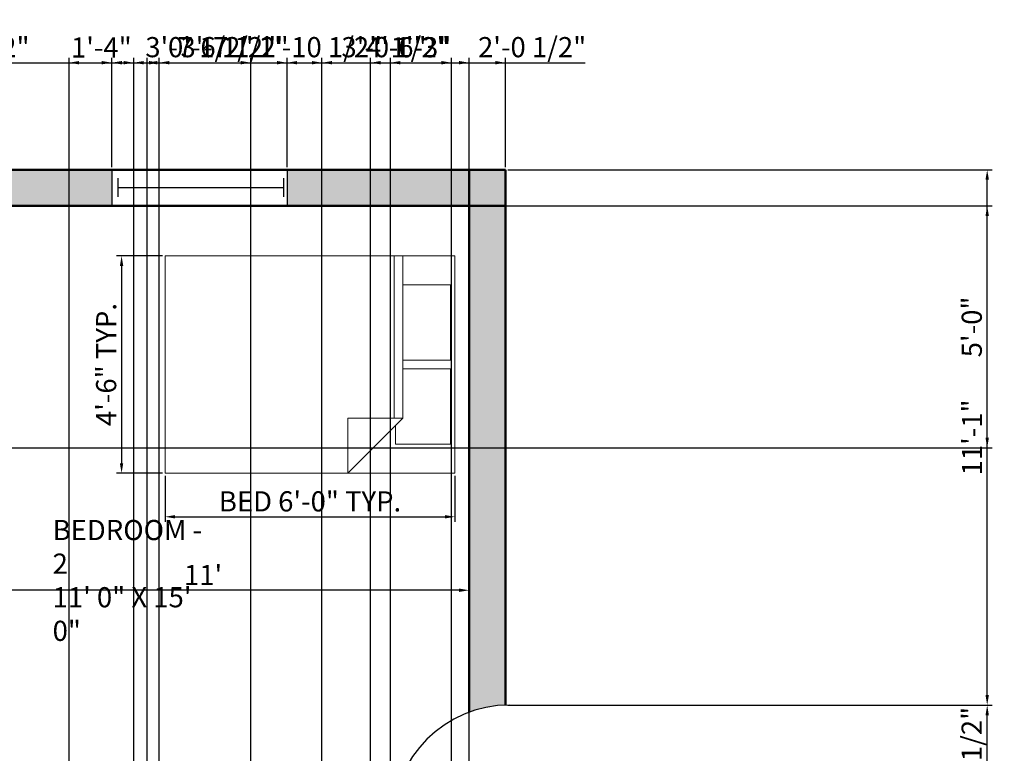
# Model space of a CAD drawing. Units: millimetres. Extents: x 2976 to 3516, y 849 to 1445.
# Tile 7 of 7: x 3272 to 3516, y 1263 to 1445. Entities that reach past the tile are written whole.
import ezdxf

# ---------------------------------------------------------------- set-up
doc = ezdxf.new("R2010")
doc.units = ezdxf.units.MM
for name, color, linetype, lineweight in [('A-AREA-IDEN', 150, 'Continuous', 25), ('A-WALL-PATT', 3, 'Continuous', 13), ('dimensions', 50, 'Continuous', 18), ('doors', 190, 'Continuous', 25), ('furniture', 130, 'Continuous', 18), ('walls', 80, 'Continuous', 50), ('windows', 10, 'Continuous', 25)]:
    doc.layers.add(name, color=color, linetype=linetype, lineweight=lineweight)
doc.styles.get("Standard").update_dxf_attribs({"font": 'arial.ttf'})
doc.dimstyles.new('ISO-25', dxfattribs={"dimtxt": 5, "dimasz": 2.5, "dimexe": 1.25, "dimexo": 0.625, "dimtad": 1, "dimdec": 0, "dimlunit": 3, "dimtxsty": 'Standard', "dimcen": 2.5, "dimadec": 0, "dimazin": 0, "dimtfac": 1, "dimtdec": 0, "dimtmove": 0, "dimatfit": 3, "dimfxl": 1, "dimarcsym": 0})

# ---------------------------------------------------------------- blocks, each defined once
blk = doc.blocks.new('*U2')
for p, q in [((0, 0), (0, -6)), ((40, 0), (40, -6))]:
    blk.add_line(p, q)
blk.add_lwpolyline([(0, 0), (0, 40), (1.75, 40), (1.75, 0)], close=True)
blk.add_arc((0, 0), 40, 0, 90)
blk = doc.blocks.new('*U4')
for p, q in [((0, 4), (0, 0)), ((36, 4), (36, 0)), ((0, 2), (36, 2))]:
    blk.add_line(p, q)
blk = doc.blocks.new('Bed - Queen')
for p, q in [((0, -80.00003), (0, 0)), ((0, 0), (59.99999, 0)), ((59.99999, 0), (59.99999, -80.00003)), ((7.99999, -1.2), (28.79998, -1.2)), ((7.99999, -14.4), (7.99999, -1.2)), ((28.79998, -1.2), (28.79998, -14.4)), ((31.19999, -1.2), (51.99999, -1.2)), ((31.19999, -14.4), (31.19999, -1.2)), ((51.99999, -1.2), (51.99999, -16.4)), ((0, -14.4), (44.8, -14.4)), ((59.99999, -29.6), (44.8, -14.4)), ((44.8, -14.4), (44.8, -29.6)), ((44.8, -16.8), (0, -16.8)), ((51.99999, -16.4), (46.79936, -16.4)), ((44.8, -29.6), (59.99999, -29.6)), ((59.99999, -80.00003), (0, -80.00003))]:
    blk.add_line(p, q)
blk = doc.blocks.new('*D13')
at = {"layer": 'Defpoints', "color": 0, "transparency": 16777216}
for p in [(3251.67, 1303.56), (3251.67, 1303.56), (3383.67, 1303.56)]:
    blk.add_point(p, dxfattribs=at)
at = {"layer": 'dimensions', "color": 0, "lineweight": -2, "transparency": 16777216}
for p, q in [((3251.67, 1304.18), (3251.67, 1304.81)), ((3383.67, 1304.18), (3383.67, 1304.81)), ((3381.17, 1303.56), (3254.17, 1303.56))]:
    blk.add_line(p, q, dxfattribs=at)
at = {"layer": 'dimensions', "color": 0, "transparency": 16777216}
for points in [[(3254.17, 1303.98), (3254.17, 1303.14), (3251.67, 1303.56)], [(3381.17, 1303.98), (3381.17, 1303.14), (3383.67, 1303.56)]]:
    blk.add_solid(points, dxfattribs=at)
at = {"layer": 'dimensions', "color": 0, "transparency": 16777216, "insert": (3317.67, 1306.69), "char_height": 5, "attachment_point": 5}
blk.add_mtext("11'", dxfattribs=at)
blk = doc.blocks.new('*D30')
at = {"layer": 'Defpoints', "color": 0, "transparency": 16777216}
for p in [(3308.23, 1332.58), (3380.16, 1332.58), (3380.16, 1321.79)]:
    blk.add_point(p, dxfattribs=at)
at = {"layer": 'dimensions', "color": 0, "lineweight": -2, "transparency": 16777216}
for p, q in [((3308.23, 1331.95), (3308.23, 1320.54)), ((3380.16, 1331.95), (3380.16, 1320.54)), ((3310.73, 1321.79), (3377.66, 1321.79))]:
    blk.add_line(p, q, dxfattribs=at)
at = {"layer": 'dimensions', "color": 0, "transparency": 16777216}
for points in [[(3310.73, 1322.2), (3310.73, 1321.37), (3308.23, 1321.79)], [(3377.66, 1322.2), (3377.66, 1321.37), (3380.16, 1321.79)]]:
    blk.add_solid(points, dxfattribs=at)
at = {"layer": 'dimensions', "color": 0, "transparency": 16777216, "insert": (3344.2, 1324.96), "char_height": 5, "attachment_point": 5}
blk.add_mtext('BED 6\'-0" TYP.', dxfattribs=at)
blk = doc.blocks.new('*D31')
at = {"layer": 'Defpoints', "color": 0, "transparency": 16777216}
for p in [(3308.23, 1386.52), (3297.45, 1332.58), (3308.23, 1332.58)]:
    blk.add_point(p, dxfattribs=at)
at = {"layer": 'dimensions', "color": 0, "lineweight": -2, "transparency": 16777216}
for p, q in [((3307.61, 1386.52), (3296.2, 1386.52)), ((3297.45, 1384.02), (3297.45, 1335.08)), ((3307.61, 1332.58), (3296.2, 1332.58))]:
    blk.add_line(p, q, dxfattribs=at)
at = {"layer": 'dimensions', "color": 0, "transparency": 16777216}
for points in [[(3297.03, 1384.02), (3297.86, 1384.02), (3297.45, 1386.52)], [(3297.03, 1335.08), (3297.86, 1335.08), (3297.45, 1332.58)]]:
    blk.add_solid(points, dxfattribs=at)
at = {"layer": 'dimensions', "color": 0, "transparency": 16777216, "insert": (3294.27, 1359.55), "char_height": 5, "attachment_point": 5, "rotation": 90}
blk.add_mtext('4\'-6" TYP.', dxfattribs=at)
blk = doc.blocks.new('*D40')
at = {"layer": 'Defpoints', "color": 0, "transparency": 16777216}
for p in [(3392.67, 1407.88), (3512.21, 1407.88), (3392.67, 1275.07)]:
    blk.add_point(p, dxfattribs=at)
at = {"layer": 'dimensions', "color": 0, "lineweight": -2, "transparency": 16777216}
for p, q in [((3393.3, 1407.88), (3513.46, 1407.88)), ((3512.21, 1277.57), (3512.21, 1405.38)), ((3393.3, 1275.07), (3513.46, 1275.07))]:
    blk.add_line(p, q, dxfattribs=at)
at = {"layer": 'dimensions', "color": 0, "transparency": 16777216}
for points in [[(3511.79, 1405.38), (3512.63, 1405.38), (3512.21, 1407.88)], [(3511.79, 1277.57), (3512.63, 1277.57), (3512.21, 1275.07)]]:
    blk.add_solid(points, dxfattribs=at)
at = {"layer": 'dimensions', "color": 0, "transparency": 16777216, "insert": (3509.08, 1341.47), "char_height": 5, "attachment_point": 5, "rotation": 90}
blk.add_mtext('11\'-1"', dxfattribs=at)
blk = doc.blocks.new('*D49')
at = {"layer": 'Defpoints', "color": 0, "transparency": 16777216}
for p in [(3295.02, 1434.42), (3223.57, 1407.88), (3295.02, 1407.88)]:
    blk.add_point(p, dxfattribs=at)
at = {"layer": 'dimensions', "color": 0, "lineweight": -2, "transparency": 16777216}
for p, q in [((3223.57, 1408.51), (3223.57, 1435.67)), ((3226.07, 1434.42), (3292.52, 1434.42)), ((3295.02, 1408.51), (3295.02, 1435.67))]:
    blk.add_line(p, q, dxfattribs=at)
at = {"layer": 'dimensions', "color": 0, "transparency": 16777216}
for points in [[(3226.07, 1434.84), (3226.07, 1434), (3223.57, 1434.42)], [(3292.52, 1434.84), (3292.52, 1434), (3295.02, 1434.42)]]:
    blk.add_solid(points, dxfattribs=at)
at = {"layer": 'dimensions', "color": 0, "transparency": 16777216, "insert": (3259.3, 1437.63), "char_height": 5, "attachment_point": 5}
blk.add_mtext('5\'-11 1/2"', dxfattribs=at)
blk = doc.blocks.new('*D50')
at = {"layer": 'Defpoints', "color": 0, "transparency": 16777216}
for p in [(3338.5, 1434.42), (3295.02, 1407.88), (3338.5, 1407.88)]:
    blk.add_point(p, dxfattribs=at)
at = {"layer": 'dimensions', "color": 0, "lineweight": -2, "transparency": 16777216}
for p, q in [((3295.02, 1408.51), (3295.02, 1435.67)), ((3297.52, 1434.42), (3336, 1434.42)), ((3338.5, 1408.51), (3338.5, 1435.67))]:
    blk.add_line(p, q, dxfattribs=at)
at = {"layer": 'dimensions', "color": 0, "transparency": 16777216}
for points in [[(3297.52, 1434.84), (3297.52, 1434), (3295.02, 1434.42)], [(3336, 1434.84), (3336, 1434), (3338.5, 1434.42)]]:
    blk.add_solid(points, dxfattribs=at)
at = {"layer": 'dimensions', "color": 0, "transparency": 16777216, "insert": (3316.76, 1437.63), "char_height": 5, "attachment_point": 5}
blk.add_mtext('3\'-7 1/2"', dxfattribs=at)
blk = doc.blocks.new('*D51')
at = {"layer": 'Defpoints', "color": 0, "transparency": 16777216}
for p in [(3392.67, 1434.42), (3338.5, 1407.88), (3392.67, 1407.88)]:
    blk.add_point(p, dxfattribs=at)
at = {"layer": 'dimensions', "color": 0, "lineweight": -2, "transparency": 16777216}
for p, q in [((3338.5, 1408.51), (3338.5, 1435.67)), ((3341, 1434.42), (3390.17, 1434.42)), ((3392.67, 1408.51), (3392.67, 1435.67))]:
    blk.add_line(p, q, dxfattribs=at)
at = {"layer": 'dimensions', "color": 0, "transparency": 16777216}
for points in [[(3341, 1434.84), (3341, 1434), (3338.5, 1434.42)], [(3390.17, 1434.84), (3390.17, 1434), (3392.67, 1434.42)]]:
    blk.add_solid(points, dxfattribs=at)
at = {"layer": 'dimensions', "color": 0, "transparency": 16777216, "insert": (3365.58, 1437.6), "char_height": 5, "attachment_point": 5}
blk.add_mtext('4\'-6"', dxfattribs=at)
blk = doc.blocks.new('*D55')
at = {"layer": 'Defpoints', "color": 0, "transparency": 16777216}
for p in [(3300.46, 1434.42), (3284.41, 1083.88), (3300.46, 1083.88)]:
    blk.add_point(p, dxfattribs=at)
at = {"layer": 'dimensions', "color": 0, "lineweight": -2, "transparency": 16777216}
for p, q in [((3284.41, 1084.51), (3284.41, 1435.67)), ((3286.91, 1434.42), (3297.96, 1434.42)), ((3300.46, 1084.51), (3300.46, 1435.67))]:
    blk.add_line(p, q, dxfattribs=at)
at = {"layer": 'dimensions', "color": 0, "transparency": 16777216}
for points in [[(3286.91, 1434.84), (3286.91, 1434), (3284.41, 1434.42)], [(3297.96, 1434.84), (3297.96, 1434), (3300.46, 1434.42)]]:
    blk.add_solid(points, dxfattribs=at)
at = {"layer": 'dimensions', "color": 0, "transparency": 16777216, "insert": (3292.43, 1437.56), "char_height": 5, "attachment_point": 5}
blk.add_mtext('1\'-4"', dxfattribs=at)
blk = doc.blocks.new('*D56')
at = {"layer": 'Defpoints', "color": 0, "transparency": 16777216}
for p in [(3392.67, 1275.07), (3512.21, 1275.07), (3392.67, 1247.37)]:
    blk.add_point(p, dxfattribs=at)
at = {"layer": 'dimensions', "color": 0, "lineweight": -2, "transparency": 16777216}
for p, q in [((3393.3, 1275.07), (3513.46, 1275.07)), ((3512.21, 1249.87), (3512.21, 1272.57)), ((3393.3, 1247.37), (3513.46, 1247.37))]:
    blk.add_line(p, q, dxfattribs=at)
at = {"layer": 'dimensions', "color": 0, "transparency": 16777216}
for points in [[(3511.79, 1272.57), (3512.63, 1272.57), (3512.21, 1275.07)], [(3511.79, 1249.87), (3512.63, 1249.87), (3512.21, 1247.37)]]:
    blk.add_solid(points, dxfattribs=at)
at = {"layer": 'dimensions', "color": 0, "transparency": 16777216, "insert": (3509, 1261.22), "char_height": 5, "attachment_point": 5, "rotation": 90}
blk.add_mtext('2\'-3 1/2"', dxfattribs=at)
blk = doc.blocks.new('*D59')
at = {"layer": 'Defpoints', "color": 0, "transparency": 16777216}
for p in [(3347.17, 1434.42), (3303.78, 1017.88), (3347.17, 1017.88)]:
    blk.add_point(p, dxfattribs=at)
at = {"layer": 'dimensions', "color": 0, "lineweight": -2, "transparency": 16777216}
for p, q in [((3303.78, 1018.51), (3303.78, 1435.67)), ((3306.28, 1434.42), (3344.67, 1434.42)), ((3347.17, 1018.51), (3347.17, 1435.67))]:
    blk.add_line(p, q, dxfattribs=at)
at = {"layer": 'dimensions', "color": 0, "transparency": 16777216}
for points in [[(3306.28, 1434.84), (3306.28, 1434), (3303.78, 1434.42)], [(3344.67, 1434.84), (3344.67, 1434), (3347.17, 1434.42)]]:
    blk.add_solid(points, dxfattribs=at)
at = {"layer": 'dimensions', "color": 0, "transparency": 16777216, "insert": (3325.48, 1437.63), "char_height": 5, "attachment_point": 5}
blk.add_mtext('3\'-7 1/2"', dxfattribs=at)
blk = doc.blocks.new('*D61')
at = {"layer": 'Defpoints', "color": 0, "transparency": 16777216}
for p in [(3383.67, 1434.42), (3359.24, 1209.88), (3383.67, 1209.88)]:
    blk.add_point(p, dxfattribs=at)
at = {"layer": 'dimensions', "color": 0, "lineweight": -2, "transparency": 16777216}
for p, q in [((3359.24, 1210.51), (3359.24, 1435.67)), ((3361.74, 1434.42), (3381.17, 1434.42)), ((3383.67, 1210.51), (3383.67, 1435.67)), ((3383.67, 1434.42), (3412.45, 1434.42))]:
    blk.add_line(p, q, dxfattribs=at)
at = {"layer": 'dimensions', "color": 0, "transparency": 16777216}
for points in [[(3361.74, 1434.84), (3361.74, 1434), (3359.24, 1434.42)], [(3381.17, 1434.84), (3381.17, 1434), (3383.67, 1434.42)]]:
    blk.add_solid(points, dxfattribs=at)
at = {"layer": 'dimensions', "color": 0, "transparency": 16777216, "insert": (3399.31, 1437.63), "char_height": 5, "attachment_point": 5}
blk.add_mtext('2\'-0 1/2"', dxfattribs=at)
blk = doc.blocks.new('*D62')
at = {"layer": 'Defpoints', "color": 0, "transparency": 16777216}
for p in [(3379.31, 1434.42), (3364.14, 1196.55), (3379.31, 1196.55)]:
    blk.add_point(p, dxfattribs=at)
at = {"layer": 'dimensions', "color": 0, "lineweight": -2, "transparency": 16777216}
for p, q in [((3364.14, 1197.18), (3364.14, 1435.67)), ((3366.64, 1434.42), (3376.81, 1434.42)), ((3379.31, 1197.18), (3379.31, 1435.67))]:
    blk.add_line(p, q, dxfattribs=at)
at = {"layer": 'dimensions', "color": 0, "transparency": 16777216}
for points in [[(3366.64, 1434.84), (3366.64, 1434), (3364.14, 1434.42)], [(3376.81, 1434.84), (3376.81, 1434), (3379.31, 1434.42)]]:
    blk.add_solid(points, dxfattribs=at)
at = {"layer": 'dimensions', "color": 0, "transparency": 16777216, "insert": (3371.72, 1437.6), "char_height": 5, "attachment_point": 5}
blk.add_mtext('1\'-3"', dxfattribs=at)
blk = doc.blocks.new('*D65')
at = {"layer": 'Defpoints', "color": 0, "transparency": 16777216}
for p in [(3329.5, 1434.42), (3306.79, 1105.27), (3329.5, 1105.27)]:
    blk.add_point(p, dxfattribs=at)
at = {"layer": 'dimensions', "color": 0, "lineweight": -2, "transparency": 16777216}
for p, q in [((3306.79, 1105.89), (3306.79, 1435.67)), ((3309.29, 1434.42), (3327, 1434.42)), ((3329.5, 1105.89), (3329.5, 1435.67)), ((3329.5, 1434.42), (3361.61, 1434.42))]:
    blk.add_line(p, q, dxfattribs=at)
at = {"layer": 'dimensions', "color": 0, "transparency": 16777216}
for points in [[(3309.29, 1434.84), (3309.29, 1434), (3306.79, 1434.42)], [(3327, 1434.84), (3327, 1434), (3329.5, 1434.42)]]:
    blk.add_solid(points, dxfattribs=at)
at = {"layer": 'dimensions', "color": 0, "transparency": 16777216, "insert": (3346.8, 1437.63), "char_height": 5, "attachment_point": 5}
blk.add_mtext('1\'-10 1/2"', dxfattribs=at)
blk = doc.blocks.new('*D69')
at = {"layer": 'Defpoints', "color": 0, "transparency": 16777216}
for p in [(3306.79, 1434.42), (3300.46, 1108.35), (3306.79, 1105.27)]:
    blk.add_point(p, dxfattribs=at)
at = {"layer": 'dimensions', "color": 0, "lineweight": -2, "transparency": 16777216}
for p, q in [((3300.46, 1108.97), (3300.46, 1435.67)), ((3302.96, 1434.42), (3304.29, 1434.42)), ((3306.79, 1105.89), (3306.79, 1435.67)), ((3306.79, 1434.42), (3335.48, 1434.42))]:
    blk.add_line(p, q, dxfattribs=at)
at = {"layer": 'dimensions', "color": 0, "transparency": 16777216}
for points in [[(3302.96, 1434.84), (3302.96, 1434), (3300.46, 1434.42)], [(3304.29, 1434.84), (3304.29, 1434), (3306.79, 1434.42)]]:
    blk.add_solid(points, dxfattribs=at)
at = {"layer": 'dimensions', "color": 0, "transparency": 16777216, "insert": (3322.39, 1437.63), "char_height": 5, "attachment_point": 5}
blk.add_mtext('0\'-6 1/2"', dxfattribs=at)
blk = doc.blocks.new('*D76')
at = {"layer": 'Defpoints', "color": 0, "transparency": 16777216}
for p in [(3051.83, 1398.88), (3512.21, 1398.88), (3051.83, 1338.88)]:
    blk.add_point(p, dxfattribs=at)
at = {"layer": 'dimensions', "color": 0, "lineweight": -2, "transparency": 16777216}
for p, q in [((3052.46, 1398.88), (3513.46, 1398.88)), ((3512.21, 1341.38), (3512.21, 1396.38)), ((3052.46, 1338.88), (3513.46, 1338.88))]:
    blk.add_line(p, q, dxfattribs=at)
at = {"layer": 'dimensions', "color": 0, "transparency": 16777216}
for points in [[(3511.79, 1396.38), (3512.63, 1396.38), (3512.21, 1398.88)], [(3511.79, 1341.38), (3512.63, 1341.38), (3512.21, 1338.88)]]:
    blk.add_solid(points, dxfattribs=at)
at = {"layer": 'dimensions', "color": 0, "transparency": 16777216, "insert": (3509.03, 1368.88), "char_height": 5, "attachment_point": 5, "rotation": 90}
blk.add_mtext('5\'-0"', dxfattribs=at)
blk = doc.blocks.new('*D80')
at = {"layer": 'Defpoints', "color": 0, "transparency": 16777216}
for p in [(3383.67, 1434.42), (3347.17, 1017.88), (3383.67, 1008.88)]:
    blk.add_point(p, dxfattribs=at)
at = {"layer": 'dimensions', "color": 0, "lineweight": -2, "transparency": 16777216}
for p, q in [((3347.17, 1018.51), (3347.17, 1435.67)), ((3349.67, 1434.42), (3381.17, 1434.42)), ((3383.67, 1009.51), (3383.67, 1435.67))]:
    blk.add_line(p, q, dxfattribs=at)
at = {"layer": 'dimensions', "color": 0, "transparency": 16777216}
for points in [[(3349.67, 1434.84), (3349.67, 1434), (3347.17, 1434.42)], [(3381.17, 1434.84), (3381.17, 1434), (3383.67, 1434.42)]]:
    blk.add_solid(points, dxfattribs=at)
at = {"layer": 'dimensions', "color": 0, "transparency": 16777216, "insert": (3365.42, 1437.63), "char_height": 5, "attachment_point": 5}
blk.add_mtext('3\'-0 1/2"', dxfattribs=at)

msp = doc.modelspace()

# ---------------------------------------------------------------- hatches: boundary and pattern name
at = {"layer": 'A-WALL-PATT'}
h = msp.add_hatch(color=256, dxfattribs=at)
h.dxf.hatch_style = 1
h.paths.add_polyline_path([(3022.67, 1398.88), (3013.67, 1398.88), (3013.67, 1278.88), (3022.67, 1278.88)])
h.paths.add_polyline_path([(3082.67, 1278.88), (3022.67, 1278.88), (3022.67, 1269.88), (3082.67, 1269.88)])
h.paths.add_polyline_path([(3022.67, 1278.88), (3013.67, 1278.88), (3013.67, 1269.88), (3022.67, 1269.88)])
h.paths.add_polyline_path([(3091.67, 1278.88), (3082.67, 1278.88), (3082.67, 1269.88), (3091.67, 1269.88)])
h.paths.add_polyline_path([(3121.76, 1278.88), (3091.67, 1278.88), (3091.67, 1269.88), (3121.76, 1269.88), (3121.76, 1272.56)])
h.paths.add_polyline_path([(3022.67, 1269.88), (3013.67, 1269.88), (3013.67, 1149.88), (3022.67, 1149.88)])
h.paths.add_polyline_path([(3022.67, 1140.88), (3013.67, 1140.88), (3013.67, 1017.88), (3022.67, 1017.88)])
h.paths.add_polyline_path([(3022.67, 1149.88), (3013.67, 1149.88), (3013.67, 1140.88), (3022.67, 1140.88)])
h.paths.add_polyline_path([(3082.67, 1149.88), (3022.67, 1149.88), (3022.67, 1140.88), (3082.67, 1140.88)])
h.paths.add_polyline_path([(3091.67, 1149.88), (3082.67, 1149.88), (3082.67, 1140.88), (3091.67, 1140.88)])
h.paths.add_polyline_path([(3143.42, 1147.68), (3143.42, 1149.88), (3091.67, 1149.88), (3091.67, 1140.88), (3144.23, 1140.88, -0.059251)])
h.paths.add_polyline_path([(3193.67, 1149.88), (3172.4, 1149.88), (3172.4, 1147.68), (3172.4, 1140.88), (3193.67, 1140.88)])
h.paths.add_polyline_path([(3202.67, 1149.88), (3193.67, 1149.88), (3193.67, 1140.88), (3202.67, 1140.88)])
h.paths.add_polyline_path([(3272.67, 1149.88), (3262.67, 1149.88), (3262.67, 1140.88), (3272.67, 1140.88)])
h.paths.add_polyline_path([(3272.67, 1140.88), (3262.67, 1140.88), (3262.67, 1083.88), (3272.67, 1083.88)])
h.paths.add_polyline_path([(3202.67, 1140.88), (3193.67, 1140.88), (3193.67, 1090.58), (3195.4, 1090.58, -0.118064), (3202.67, 1088.84)])
h.paths.add_polyline_path([(3202.67, 1074.53), (3195.4, 1074.53), (3193.67, 1074.53), (3193.67, 1017.88), (3202.67, 1017.88)])
h.paths.add_polyline_path([(3202.67, 1017.88), (3193.67, 1017.88), (3193.67, 1008.88), (3202.67, 1008.88)])
h.paths.add_polyline_path([(3193.67, 1017.88), (3112.23, 1017.88), (3112.23, 1008.88), (3193.67, 1008.88)])
h.paths.add_polyline_path([(3068.25, 1017.88), (3022.67, 1017.88), (3022.67, 1008.88), (3068.25, 1008.88)])
h.paths.add_polyline_path([(3022.67, 1017.88), (3013.67, 1017.88), (3013.67, 1008.88), (3022.67, 1008.88)])
h.paths.add_polyline_path([(3272.67, 1074.88), (3262.67, 1074.88), (3262.67, 1017.88), (3271.67, 1017.88), (3272.67, 1017.88)])
h.paths.add_polyline_path([(3272.67, 1083.88), (3262.67, 1083.88), (3262.67, 1074.88), (3272.67, 1074.88)])
h.paths.add_polyline_path([(3284.41, 1082.91), (3284.41, 1083.88), (3272.67, 1083.88), (3272.67, 1074.88), (3284.41, 1074.88)])
h.paths.add_polyline_path([(3383.67, 1083.88), (3300.46, 1083.88), (3300.46, 1082.91, -0.131652), (3298.31, 1074.88), (3383.67, 1074.88)])
h.paths.add_polyline_path([(3392.67, 1083.88), (3383.67, 1083.88), (3383.67, 1074.88), (3392.67, 1074.88)])
h.paths.add_polyline_path([(3392.67, 1074.88), (3383.67, 1074.88), (3383.67, 1017.88), (3392.67, 1017.88)])
h.paths.add_polyline_path([(3392.67, 1017.88), (3383.67, 1017.88), (3383.67, 1008.88), (3392.67, 1008.88)])
h.paths.add_polyline_path([(3383.67, 1017.88), (3347.17, 1017.88), (3347.17, 1008.88), (3383.67, 1008.88)])
h.paths.add_polyline_path([(3303.78, 1017.88), (3272.67, 1017.88), (3272.67, 1008.88), (3303.78, 1008.88)])
h.paths.add_polyline_path([(3272.67, 1017.88), (3271.67, 1017.88), (3262.67, 1017.88), (3262.67, 1008.88), (3272.67, 1008.88)])
h.paths.add_polyline_path([(3262.67, 1017.88), (3243.44, 1017.88), (3243.44, 1008.88), (3262.67, 1008.88)])
h.paths.add_polyline_path([(3218.58, 1017.88), (3202.67, 1017.88), (3202.67, 1008.88), (3218.58, 1008.88)])
h.paths.add_polyline_path([(3392.67, 1209.88), (3383.67, 1209.88), (3383.67, 1083.88), (3392.67, 1083.88)])
h.paths.add_polyline_path([(3392.67, 1218.88), (3383.67, 1218.88), (3383.67, 1209.88), (3392.67, 1209.88)])
h.paths.add_polyline_path([(3392.67, 1246.1), (3383.67, 1246.1), (3383.67, 1218.88), (3392.67, 1218.88)])
h.paths.add_polyline_path([(3383.67, 1218.88), (3251.67, 1218.88), (3251.67, 1209.88), (3383.67, 1209.88)])
h.paths.add_polyline_path([(3251.67, 1287.88), (3242.67, 1287.88), (3242.67, 1218.88), (3251.67, 1218.88)])
h.paths.add_polyline_path([(3251.67, 1218.88), (3242.67, 1218.88), (3242.67, 1209.88), (3251.67, 1209.88)])
h.paths.add_polyline_path([(3251.67, 1398.88), (3242.67, 1398.88), (3242.67, 1296.88), (3251.67, 1296.88)])
h.paths.add_polyline_path([(3251.67, 1296.88), (3242.67, 1296.88), (3242.67, 1287.88), (3251.67, 1287.88)])
h.paths.add_polyline_path([(3242.67, 1296.88), (3182.67, 1296.88), (3182.67, 1287.88), (3242.67, 1287.88)])
h.paths.add_polyline_path([(3182.67, 1296.88), (3173.67, 1296.88), (3173.67, 1287.88), (3182.67, 1287.88)])
h.paths.add_polyline_path([(3182.67, 1287.88), (3173.67, 1287.88), (3173.67, 1278.88), (3182.67, 1278.88)])
h.paths.add_polyline_path([(3182.67, 1278.88), (3173.67, 1278.88), (3173.67, 1269.88), (3182.67, 1269.88)])
h.paths.add_polyline_path([(3173.67, 1278.88), (3150.05, 1278.88, -0.054989), (3150.74, 1272.56), (3150.74, 1269.88), (3173.67, 1269.88)])
h.paths.add_polyline_path([(3182.67, 1398.88), (3173.67, 1398.88), (3173.67, 1296.88), (3182.67, 1296.88)])
h.paths.add_polyline_path([(3182.67, 1407.88), (3173.67, 1407.88), (3173.67, 1398.88), (3182.67, 1398.88)])
h.paths.add_polyline_path([(3173.67, 1407.88), (3104.59, 1407.88), (3104.59, 1398.88), (3173.67, 1398.88)])
h.paths.add_polyline_path([(3060.33, 1407.88), (3022.67, 1407.88), (3022.67, 1398.88), (3060.33, 1398.88)])
h.paths.add_polyline_path([(3022.67, 1407.88), (3013.67, 1407.88), (3013.67, 1398.88), (3022.67, 1398.88)])
h.paths.add_polyline_path([(3196.7, 1407.88), (3182.67, 1407.88), (3182.67, 1398.88), (3196.7, 1398.88)])
h.paths.add_polyline_path([(3242.67, 1407.88), (3223.57, 1407.88), (3223.57, 1398.88), (3242.67, 1398.88)])
h.paths.add_polyline_path([(3251.67, 1407.88), (3242.67, 1407.88), (3242.67, 1398.88), (3251.67, 1398.88)])
h.paths.add_polyline_path([(3295.02, 1407.88), (3251.67, 1407.88), (3251.67, 1398.88), (3295.02, 1398.88)])
h.paths.add_polyline_path([(3383.67, 1407.88), (3338.5, 1407.88), (3338.5, 1398.88), (3383.67, 1398.88)])
h.paths.add_polyline_path([(3392.67, 1407.88), (3383.67, 1407.88), (3383.67, 1398.88), (3392.67, 1398.88)])
h.paths.add_polyline_path([(3392.67, 1398.88), (3383.67, 1398.88), (3383.67, 1273.3, -0.079613), (3392.67, 1275.07)])

# ---------------------------------------------------------------- linework, layer by layer
at = {"layer": 'walls'}
for p, q in [((3013.67, 1407.88), (3392.67, 1407.88)), ((3383.67, 1407.88), (3383.67, 1273.3)), ((3392.67, 1407.88), (3392.67, 1275.07)), ((3013.67, 1398.88), (3392.67, 1398.88))]:
    msp.add_line(p, q, dxfattribs=at)
at = {"layer": 'windows'}
for p, q in [((3295.02, 1407.88), (3295.02, 1398.88)), ((3338.5, 1407.88), (3338.5, 1398.88))]:
    msp.add_line(p, q, dxfattribs=at)

# ---------------------------------------------------------------- block references
at = {"layer": 'doors', "xscale": 0.7246062005204927, "yscale": 0.7246062005204927, "zscale": 0.7246062005204927, "rotation": 90}
msp.add_blockref('*U2', (3393.69, 1246.1), dxfattribs=at)
at = {"layer": 'furniture', "xscale": 0.8990276149147879, "yscale": 0.8990276149147879, "zscale": 0.8990276149147879, "rotation": 270}
msp.add_blockref('Bed - Queen', (3380.16, 1386.52), dxfattribs=at)
at = {"layer": 'windows', "xscale": 1.141608635997284, "yscale": 1.141608635997284, "zscale": 1.141608635997284}
msp.add_blockref('*U4', (3296.52, 1401.18), dxfattribs=at)

# ---------------------------------------------------------------- texts
at = {"layer": 'A-AREA-IDEN', "insert": (3280.34, 1321), "char_height": 5, "attachment_point": 1}
msp.add_mtext_dynamic_manual_height_columns('BEDROOM - 2 \\P11\' 0" X 15\' 0"', width=38.078, gutter_width=12.5, heights=[0], dxfattribs=at)

# ---------------------------------------------------------------- dimensions: what is measured, and where the dimension line sits
at = {"layer": 'dimensions'}
for base, p1, p2, override, picture, middle in [((3295.0222, 1434.4215), (3223.5747, 1407.8815), (3295.0222, 1407.8815), {"dimdec": 1, "dimlfac": 1, "dimrnd": 0, "dimzin": 1, "dimdsep": 46, "dimlunit": 4, "dimfrac": 2}, '*D49', (3259.2985, 1437.6317)), ((3338.5, 1434.42), (3295.02, 1407.88), (3338.5, 1407.88), {"dimdec": 1, "dimlfac": 1, "dimrnd": 0, "dimzin": 1, "dimdsep": 46, "dimlunit": 4, "dimfrac": 2}, '*D50', (3316.76, 1437.63)), ((3306.79, 1434.42), (3300.46, 1108.35), (3306.79, 1105.27), {"dimdec": 1, "dimlfac": 1, "dimrnd": 0, "dimzin": 1, "dimdsep": 46, "dimlunit": 4, "dimfrac": 2}, '*D69', (3322.39, 1437.63)), ((3347.17, 1434.42), (3303.78, 1017.88), (3347.17, 1017.88), {"dimdec": 1, "dimlfac": 1, "dimrnd": 0, "dimzin": 1, "dimdsep": 46, "dimlunit": 4, "dimfrac": 2}, '*D59', (3325.48, 1437.63)), ((3329.5, 1434.42), (3306.79, 1105.27), (3329.5, 1105.27), {"dimdec": 1, "dimlfac": 1, "dimrnd": 0, "dimzin": 1, "dimdsep": 46, "dimlunit": 4, "dimfrac": 2}, '*D65', (3346.8, 1437.63)), ((3383.67, 1434.42), (3347.17, 1017.88), (3383.67, 1008.88), {"dimdec": 1, "dimlfac": 1, "dimrnd": 0, "dimzin": 1, "dimdsep": 46, "dimlunit": 4, "dimfrac": 2}, '*D80', (3365.42, 1437.63)), ((3383.67, 1434.42), (3359.24, 1209.88), (3383.67, 1209.88), {"dimdec": 1, "dimlfac": 1, "dimrnd": 0, "dimzin": 1, "dimdsep": 46, "dimlunit": 4, "dimfrac": 2}, '*D61', (3399.31, 1437.63)), ((3300.4593, 1434.4215), (3284.4052, 1083.8815), (3300.4593, 1083.8815), {"dimdec": 1, "dimlfac": 1, "dimrnd": 0, "dimzin": 1, "dimdsep": 46, "dimlunit": 4, "dimfrac": 2}, '*D55', (3292.4322, 1437.5567)), ((3392.67, 1434.42), (3338.5, 1407.88), (3392.67, 1407.88), {"dimdec": 1, "dimlfac": 1, "dimrnd": 0, "dimzin": 1, "dimdsep": 46, "dimlunit": 4, "dimfrac": 2}, '*D51', (3365.58, 1437.6)), ((3379.31, 1434.42), (3364.14, 1196.55), (3379.31, 1196.55), {"dimdec": 1, "dimlfac": 1, "dimrnd": 0, "dimzin": 1, "dimdsep": 46, "dimlunit": 4, "dimfrac": 2}, '*D62', (3371.72, 1437.6)), ((3251.67, 1303.56), (3383.67, 1303.56), (3251.67, 1303.56), {"dimclrd": 0, "dimclre": 0, "dimclrt": 0}, '*D13', (3317.67, 1306.69))]:
    dim = msp.add_linear_dim(base=base, p1=p1, p2=p2, dimstyle='ISO-25', override=override, dxfattribs=at)
    dim.commit()
    dim.dimension.update_dxf_attribs({"geometry": picture, "text_midpoint": middle})
for base, p1, p2, picture, middle in [((3512.21, 1407.88), (3392.67, 1275.07), (3392.67, 1407.88), '*D40', (3509.08, 1341.47)), ((3512.21, 1398.88), (3051.83, 1338.88), (3051.83, 1398.88), '*D76', (3509.03, 1368.88)), ((3512.21, 1275.07), (3392.67, 1247.37), (3392.67, 1275.07), '*D56', (3509, 1261.22))]:
    dim = msp.add_linear_dim(base=base, p1=p1, p2=p2, angle=90, dimstyle='ISO-25', override={"dimdec": 1, "dimlfac": 1, "dimrnd": 0, "dimzin": 1, "dimdsep": 46, "dimlunit": 4, "dimfrac": 2}, dxfattribs=at)
    dim.commit()
    dim.dimension.update_dxf_attribs({"geometry": picture, "text_midpoint": middle})
dim = msp.add_linear_dim(base=(3297.45, 1332.58), p1=(3308.23, 1386.52), p2=(3308.23, 1332.58), angle=270, text='<> TYP.', dimstyle='ISO-25', override={"dimdec": 1, "dimlfac": 1, "dimrnd": 0, "dimzin": 1, "dimdsep": 46, "dimlunit": 4, "dimfrac": 2}, dxfattribs=at)
dim.commit()
dim.dimension.update_dxf_attribs({"geometry": '*D31', "text_midpoint": (3294.27, 1359.55)})
dim = msp.add_linear_dim(base=(3380.16, 1321.79), p1=(3308.23, 1332.58), p2=(3380.16, 1332.58), text='BED <> TYP.', dimstyle='ISO-25', override={"dimdec": 1, "dimlfac": 1, "dimrnd": 0, "dimzin": 1, "dimdsep": 46, "dimlunit": 4, "dimfrac": 2}, dxfattribs=at)
dim.commit()
dim.dimension.update_dxf_attribs({"geometry": '*D30', "text_midpoint": (3344.2, 1324.96)})

doc.saveas('drawing.dxf')
